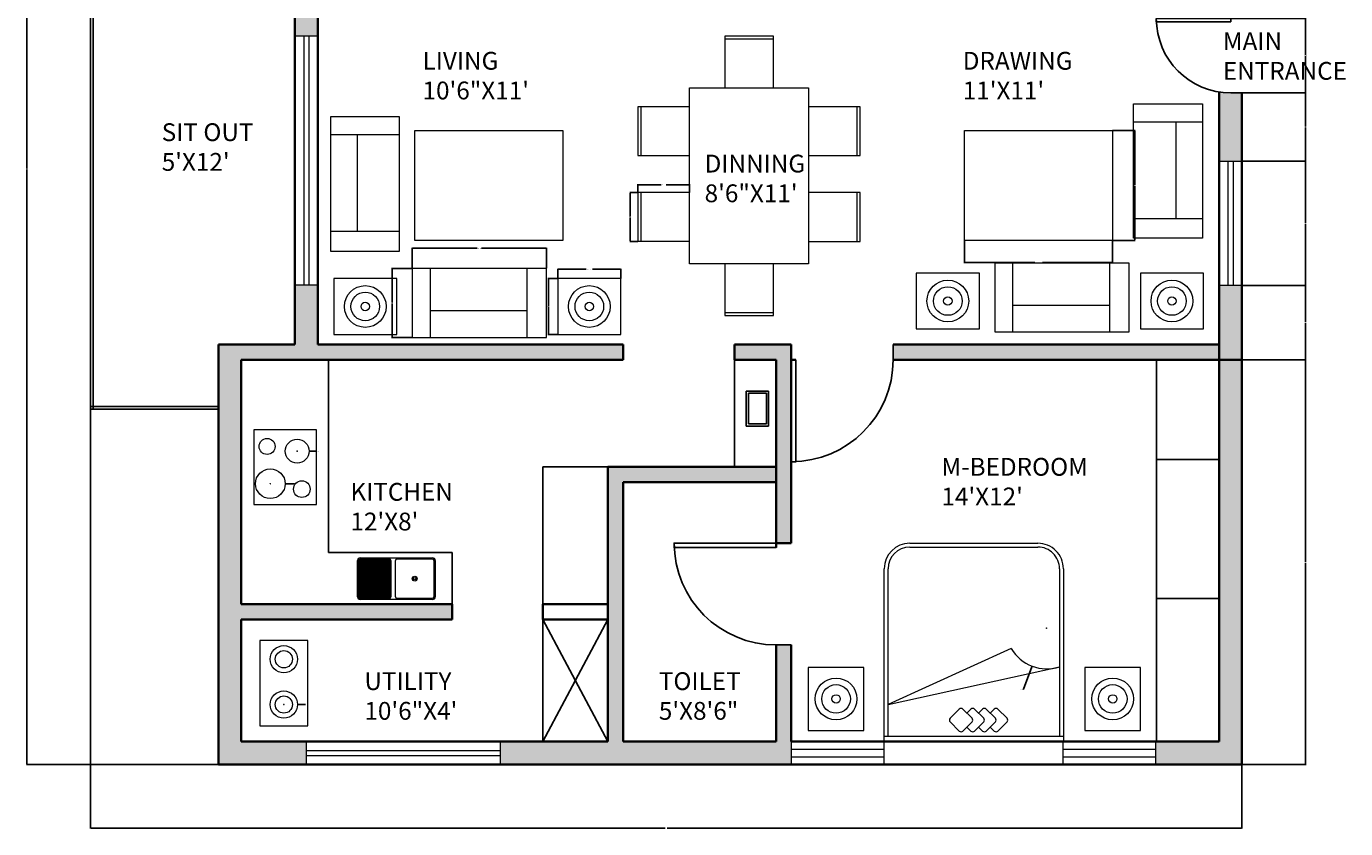
# Model space of a CAD drawing. Units: inches. Extents: x 2764 to 3282, y 1588 to 2106.
# Tile 1 of 2: x 2764 to 3282, y 1588 to 1903. Entities that reach past the tile are written whole.
import ezdxf

# ---------------------------------------------------------------- set-up
doc = ezdxf.new("R2010")
doc.units = ezdxf.units.IN
for name, color, linetype, lineweight in [('A-ANNO-DIMS', 2, 'Continuous', 18), ('A-ANNO-TEXT', 7, 'Continuous', 25), ('A-AREA-IDEN', 7, 'Continuous', 25), ('A-DOOR', 3, 'Continuous', 25), ('A-EQPM', 8, 'Continuous', 18), ('A-FIXT-PATT', 9, 'Continuous', 13), ('A-FLOR-CASE', 8, 'Continuous', 25), ('A-FLOR-FIXT', 9, 'Continuous', 18), ('A-FLOR-HRAL', 7, 'Continuous', 25), ('A-FURN', 8, 'Continuous', 18), ('A-GLAZ', 4, 'Continuous', 18), ('A-WALL', 7, 'Continuous', 35), ('A-WALL-PATT', 9, 'Continuous', 13)]:
    doc.layers.add(name, color=color, linetype=linetype, lineweight=lineweight)
doc.styles.get("Standard").update_dxf_attribs({"font": 'arial.ttf'})
doc.dimstyles.get("Standard").update_dxf_attribs({"dimtxt": 0.18, "dimasz": 0.18, "dimexe": 0.18, "dimexo": 0.0625, "dimgap": 0.09, "dimtad": 0, "dimtih": 1, "dimtoh": 1, "dimdec": 4, "dimzin": 0, "dimdsep": 46, "dimtxsty": 'Standard', "dimcen": 0.09, "dimadec": 0, "dimazin": 0, "dimtfac": 1, "dimtdec": 4, "dimtofl": 0, "dimtmove": 0, "dimatfit": 3, "dimfxl": 1, "dimtolj": 1, "dimtzin": 0, "dimarcsym": 0})

# ---------------------------------------------------------------- blocks, each defined once
blk = doc.blocks.new('*U2')
for p, q in [((0, 0), (0, -6)), ((40, 0), (40, -6))]:
    blk.add_line(p, q)
blk.add_lwpolyline([(0, 0), (0, 40), (1.75, 40), (1.75, 0)], close=True)
blk.add_arc((0, 0), 40, 0, 90)
blk = doc.blocks.new('SIDE-TABLE-WITH-LAMP')
for p, q in [((0, 21.93), (0, 0)), ((24.76, 21.93), (0, 21.93)), ((24.76, 0), (24.76, 21.93)), ((0, 0), (24.76, 0))]:
    blk.add_line(p, q)
for radius in [8.2, 5.62, 1.65]:
    blk.add_circle((12.38, 10.96), radius)
blk = doc.blocks.new('BED-DOUBLE')
for p, q in [((0, 70.34), (67.95, 70.34)), ((2.2, 70.34), (2.2, 0)), ((2.2, 68.84), (67.95, 68.84)), ((14.6, 68.84), (29.36, 1.5)), ((36.6, 20.47), (14.6, 68.84)), ((76.45, 60.34), (76.45, 10)), ((77.95, 60.34), (77.95, 10)), ((67.95, 0), (0, 0)), ((67.95, 1.5), (2.2, 1.5))]:
    blk.add_line(p, q)
blk.add_lwpolyline([(12.75, 40.88), (9.16, 44.46, 0.414214), (7.75, 44.46), (4.16, 40.88, 0.414214), (4.16, 39.46), (7.75, 35.88, 0.414214), (9.16, 35.88), (12.75, 39.46, 0.414214)], format="xyb", close=True)
for points in [[(5.75, 37.88), (4.16, 36.29, 0.414214), (4.16, 34.88), (7.75, 31.29, 0.414214), (9.16, 31.29), (12.75, 34.88, 0.414214), (12.75, 36.29), (11.16, 37.88)], [(5.75, 33.29), (4.16, 31.7, 0.414214), (4.16, 30.29), (7.75, 26.7, 0.414214), (9.16, 26.7), (12.75, 30.29, 0.414214), (12.75, 31.7), (11.16, 33.29)], [(5.75, 28.7), (4.16, 27.12, 0.414214), (4.16, 25.7), (7.75, 22.12, 0.414214), (9.16, 22.12), (12.75, 25.7, 0.414214), (12.75, 27.12), (11.16, 28.7)]]:
    blk.add_lwpolyline(points, format="xyb")
for centre, radius, start, end in [((67.95, 60.34), 10, 0, 90), ((67.95, 60.34), 8.5, 0, 90), ((44.61, 6.58), 16.03, 119.9541, 198.4829), ((67.95, 10), 10, 270, 0), ((67.95, 10), 8.5, 270, 0)]:
    blk.add_arc(centre, radius, start, end)
blk = doc.blocks.new('SOFA-TWO-SEAT')
for p, q in [((0, 27.06), (0, 0)), ((52.76, 27.06), (0, 27.06)), ((7, 27.06), (7, 0)), ((45.05, 27.06), (45.05, 0)), ((52.76, 0), (52.76, 27.06)), ((7, 10.5), (45.05, 10.5)), ((0, 0), (52.76, 0))]:
    blk.add_line(p, q)
blk = doc.blocks.new('CHAIR-DINING')
for p, q in [((20.31, 19.17), (0, 19.17)), ((0, 19.17), (0, 0)), ((1.17, 19.17), (1.17, 0)), ((0, 0), (20.31, 0))]:
    blk.add_line(p, q)
blk = doc.blocks.new('TABLE-COFFEE')
for p, q in [((0, 43.23), (58.08, 43.23)), ((0, 0), (0, 43.23)), ((58.08, 43.23), (58.08, 0)), ((58.08, 0), (0, 0))]:
    blk.add_line(p, q)
blk = doc.blocks.new('*D8')
at = {"layer": 'A-ANNO-DIMS', "color": 0, "lineweight": -2, "transparency": 16777216}
for p, q in [((2972.96, 1804.15), (2972.96, 1807.98)), ((2973.14, 1807.8), (2984.09, 1807.8)), ((2997.54, 1807.8), (2986.6, 1807.8)), ((2997.72, 1804.15), (2997.72, 1807.98))]:
    blk.add_line(p, q, dxfattribs=at)
at = {"layer": 'A-ANNO-DIMS', "color": 0, "transparency": 16777216}
for points in [[(2973.14, 1807.83), (2973.14, 1807.77), (2972.96, 1807.8)], [(2997.54, 1807.83), (2997.54, 1807.77), (2997.72, 1807.8)]]:
    blk.add_solid(points, dxfattribs=at)
at = {"layer": 'Defpoints', "color": 0, "transparency": 16777216}
for p in [(2972.96, 1804.09), (2997.72, 1807.8), (2997.72, 1804.09)]:
    blk.add_point(p, dxfattribs=at)
at = {"layer": 'A-ANNO-DIMS', "color": 0, "transparency": 16777216, "insert": (2985.34, 1807.8), "char_height": 0.18, "attachment_point": 5}
blk.add_mtext('\\A1;END TABLE 25 TYP.', dxfattribs=at)
blk = doc.blocks.new('*D9')
at = {"layer": 'A-ANNO-DIMS', "color": 0, "lineweight": -2, "transparency": 16777216}
for p, q in [((2972.9, 1804.09), (2969.07, 1804.09)), ((2969.25, 1803.91), (2969.25, 1793.31)), ((2969.25, 1782.34), (2969.25, 1792.95)), ((2972.9, 1782.16), (2969.07, 1782.16))]:
    blk.add_line(p, q, dxfattribs=at)
at = {"layer": 'A-ANNO-DIMS', "color": 0, "transparency": 16777216}
for points in [[(2969.22, 1803.91), (2969.28, 1803.91), (2969.25, 1804.09)], [(2969.22, 1782.34), (2969.28, 1782.34), (2969.25, 1782.16)]]:
    blk.add_solid(points, dxfattribs=at)
at = {"layer": 'Defpoints', "color": 0, "transparency": 16777216}
for p in [(2969.25, 1804.09), (2972.96, 1804.09), (2972.96, 1782.16)]:
    blk.add_point(p, dxfattribs=at)
at = {"layer": 'A-ANNO-DIMS', "color": 0, "transparency": 16777216, "insert": (2969.25, 1793.13), "char_height": 0.18, "attachment_point": 5}
blk.add_mtext('\\A1;22 TYP.', dxfattribs=at)
blk = doc.blocks.new('*D12')
at = {"layer": 'A-ANNO-DIMS', "color": 0, "lineweight": -2, "transparency": 16777216}
for p, q in [((3132.73, 1819.03), (3132.73, 1810.2)), ((3190.81, 1819.03), (3190.81, 1810.2)), ((3132.91, 1810.38), (3160.26, 1810.38)), ((3190.63, 1810.38), (3163.27, 1810.38))]:
    blk.add_line(p, q, dxfattribs=at)
at = {"layer": 'A-ANNO-DIMS', "color": 0, "transparency": 16777216}
for points in [[(3132.91, 1810.41), (3132.91, 1810.35), (3132.73, 1810.38)], [(3190.63, 1810.41), (3190.63, 1810.35), (3190.81, 1810.38)]]:
    blk.add_solid(points, dxfattribs=at)
at = {"layer": 'Defpoints', "color": 0, "transparency": 16777216}
for p in [(3132.73, 1819.09), (3190.81, 1819.09), (3190.81, 1810.38)]:
    blk.add_point(p, dxfattribs=at)
at = {"layer": 'A-ANNO-DIMS', "color": 0, "transparency": 16777216, "insert": (3161.77, 1810.38), "char_height": 0.18, "attachment_point": 5}
blk.add_mtext('\\A1;COFFEE TABLE 58 TYP.', dxfattribs=at)
blk = doc.blocks.new('*D13')
at = {"layer": 'A-ANNO-DIMS', "color": 0, "lineweight": -2, "transparency": 16777216}
for p, q in [((3190.87, 1862.32), (3199.7, 1862.32)), ((3199.52, 1862.14), (3199.52, 1840.89)), ((3199.52, 1819.27), (3199.52, 1840.52)), ((3190.87, 1819.09), (3199.7, 1819.09))]:
    blk.add_line(p, q, dxfattribs=at)
at = {"layer": 'A-ANNO-DIMS', "color": 0, "transparency": 16777216}
for points in [[(3199.49, 1862.14), (3199.55, 1862.14), (3199.52, 1862.32)], [(3199.49, 1819.27), (3199.55, 1819.27), (3199.52, 1819.09)]]:
    blk.add_solid(points, dxfattribs=at)
at = {"layer": 'Defpoints', "color": 0, "transparency": 16777216}
for p in [(3190.81, 1862.32), (3199.52, 1862.32), (3190.81, 1819.09)]:
    blk.add_point(p, dxfattribs=at)
at = {"layer": 'A-ANNO-DIMS', "color": 0, "transparency": 16777216, "insert": (3199.52, 1840.71), "char_height": 0.18, "attachment_point": 5}
blk.add_mtext('\\A1;43 TYP.', dxfattribs=at)
blk = doc.blocks.new('*D14')
at = {"layer": 'A-ANNO-DIMS', "color": 0, "lineweight": -2, "transparency": 16777216}
for p, q in [((2915.77, 1808.12), (2915.77, 1816.15)), ((2915.95, 1815.97), (2941.24, 1815.97)), ((2968.35, 1815.97), (2943.05, 1815.97)), ((2968.53, 1808.12), (2968.53, 1816.15))]:
    blk.add_line(p, q, dxfattribs=at)
at = {"layer": 'A-ANNO-DIMS', "color": 0, "transparency": 16777216}
for points in [[(2915.95, 1816), (2915.95, 1815.94), (2915.77, 1815.97)], [(2968.35, 1816), (2968.35, 1815.94), (2968.53, 1815.97)]]:
    blk.add_solid(points, dxfattribs=at)
at = {"layer": 'Defpoints', "color": 0, "transparency": 16777216}
for p in [(2968.53, 1815.97), (2915.77, 1808.06), (2968.53, 1808.06)]:
    blk.add_point(p, dxfattribs=at)
at = {"layer": 'A-ANNO-DIMS', "color": 0, "transparency": 16777216, "insert": (2942.15, 1815.97), "char_height": 0.18, "attachment_point": 5}
blk.add_mtext('\\A1;SOFA 53 TYP.', dxfattribs=at)
blk = doc.blocks.new('*D15')
at = {"layer": 'A-ANNO-DIMS', "color": 0, "lineweight": -2, "transparency": 16777216}
for p, q in [((2915.71, 1808.06), (2907.68, 1808.06)), ((2907.86, 1807.88), (2907.86, 1794.71)), ((2907.86, 1781.18), (2907.86, 1794.35)), ((2915.71, 1781), (2907.68, 1781))]:
    blk.add_line(p, q, dxfattribs=at)
at = {"layer": 'A-ANNO-DIMS', "color": 0, "transparency": 16777216}
for points in [[(2907.83, 1807.88), (2907.89, 1807.88), (2907.86, 1808.06)], [(2907.83, 1781.18), (2907.89, 1781.18), (2907.86, 1781)]]:
    blk.add_solid(points, dxfattribs=at)
at = {"layer": 'Defpoints', "color": 0, "transparency": 16777216}
for p in [(2907.86, 1808.06), (2915.77, 1808.06), (2915.77, 1781)]:
    blk.add_point(p, dxfattribs=at)
at = {"layer": 'A-ANNO-DIMS', "color": 0, "transparency": 16777216, "insert": (2907.86, 1794.53), "char_height": 0.18, "attachment_point": 5}
blk.add_mtext('\\A1;27 TYP.', dxfattribs=at)
blk = doc.blocks.new('*D16')
at = {"layer": 'A-ANNO-DIMS', "color": 0, "lineweight": -2, "transparency": 16777216}
for p, q in [((3004.42, 1837.95), (3004.42, 1841.12)), ((3004.6, 1840.94), (3013.62, 1840.94)), ((3024.55, 1840.94), (3015.52, 1840.94)), ((3024.73, 1837.95), (3024.73, 1841.12))]:
    blk.add_line(p, q, dxfattribs=at)
at = {"layer": 'A-ANNO-DIMS', "color": 0, "transparency": 16777216}
for points in [[(3004.6, 1840.97), (3004.6, 1840.91), (3004.42, 1840.94)], [(3024.55, 1840.97), (3024.55, 1840.91), (3024.73, 1840.94)]]:
    blk.add_solid(points, dxfattribs=at)
at = {"layer": 'Defpoints', "color": 0, "transparency": 16777216}
for p in [(3024.73, 1840.94), (3004.42, 1837.89), (3024.73, 1837.89)]:
    blk.add_point(p, dxfattribs=at)
at = {"layer": 'A-ANNO-DIMS', "color": 0, "transparency": 16777216, "insert": (3014.57, 1840.94), "char_height": 0.18, "attachment_point": 5}
blk.add_mtext('\\A1;CHAIR 20 TYP.', dxfattribs=at)
blk = doc.blocks.new('*D17')
at = {"layer": 'A-ANNO-DIMS', "color": 0, "lineweight": -2, "transparency": 16777216}
for p, q in [((3004.35, 1837.89), (3001.19, 1837.89)), ((3001.37, 1837.71), (3001.37, 1828.49)), ((3001.37, 1818.9), (3001.37, 1828.12)), ((3004.35, 1818.72), (3001.19, 1818.72))]:
    blk.add_line(p, q, dxfattribs=at)
at = {"layer": 'A-ANNO-DIMS', "color": 0, "transparency": 16777216}
for points in [[(3001.34, 1837.71), (3001.4, 1837.71), (3001.37, 1837.89)], [(3001.34, 1818.9), (3001.4, 1818.9), (3001.37, 1818.72)]]:
    blk.add_solid(points, dxfattribs=at)
at = {"layer": 'Defpoints', "color": 0, "transparency": 16777216}
for p in [(3001.37, 1837.89), (3004.42, 1837.89), (3004.42, 1818.72)]:
    blk.add_point(p, dxfattribs=at)
at = {"layer": 'A-ANNO-DIMS', "color": 0, "transparency": 16777216, "insert": (3001.37, 1828.31), "char_height": 0.18, "attachment_point": 5}
blk.add_mtext('\\A1;19 TYP.', dxfattribs=at)
blk = doc.blocks.new('*D18')
at = {"layer": 'A-ANNO-DIMS', "color": 0, "lineweight": -2, "transparency": 16777216}
for p, q in [((2789.46, 1752.72), (2789.46, 1587.96)), ((3241.66, 1613.08), (3241.66, 1587.96)), ((2789.64, 1588.14), (3015.16, 1588.14)), ((3241.48, 1588.14), (3015.96, 1588.14))]:
    blk.add_line(p, q, dxfattribs=at)
at = {"layer": 'A-ANNO-DIMS', "color": 0, "transparency": 16777216}
for points in [[(2789.64, 1588.17), (2789.64, 1588.11), (2789.46, 1588.14)], [(3241.48, 1588.17), (3241.48, 1588.11), (3241.66, 1588.14)]]:
    blk.add_solid(points, dxfattribs=at)
at = {"layer": 'Defpoints', "color": 0, "transparency": 16777216}
for p in [(2789.46, 1752.79), (3241.66, 1613.14), (3241.66, 1588.14)]:
    blk.add_point(p, dxfattribs=at)
at = {"layer": 'A-ANNO-DIMS', "color": 0, "transparency": 16777216, "insert": (3015.56, 1588.14), "char_height": 0.18, "attachment_point": 5}
blk.add_mtext('\\A1;452.2', dxfattribs=at)
blk = doc.blocks.new('*D19')
at = {"layer": 'A-ANNO-DIMS', "color": 0, "lineweight": -2, "transparency": 16777216}
for p, q in [((2839.6, 2081.14), (2764.28, 2081.14)), ((2764.46, 2080.96), (2764.46, 1847.33)), ((2764.46, 1613.32), (2764.46, 1846.96)), ((2839.6, 1613.14), (2764.28, 1613.14))]:
    blk.add_line(p, q, dxfattribs=at)
at = {"layer": 'A-ANNO-DIMS', "color": 0, "transparency": 16777216}
for points in [[(2764.43, 2080.96), (2764.49, 2080.96), (2764.46, 2081.14)], [(2764.43, 1613.32), (2764.49, 1613.32), (2764.46, 1613.14)]]:
    blk.add_solid(points, dxfattribs=at)
at = {"layer": 'Defpoints', "color": 0, "transparency": 16777216}
for p in [(2764.46, 2081.14), (2839.66, 2081.14), (2839.66, 1613.14)]:
    blk.add_point(p, dxfattribs=at)
at = {"layer": 'A-ANNO-DIMS', "color": 0, "transparency": 16777216, "insert": (2764.46, 1847.14), "char_height": 0.18, "attachment_point": 5}
blk.add_mtext('\\A1;468', dxfattribs=at)
blk = doc.blocks.new('*D30')
at = {"layer": 'A-ANNO-DIMS', "color": 0, "lineweight": -2, "transparency": 16777216}
for p, q in [((3241.72, 1772.14), (3266.84, 1772.14)), ((3266.66, 1771.96), (3266.66, 1692.83)), ((3266.66, 1613.32), (3266.66, 1692.46)), ((3241.72, 1613.14), (3266.84, 1613.14))]:
    blk.add_line(p, q, dxfattribs=at)
at = {"layer": 'A-ANNO-DIMS', "color": 0, "transparency": 16777216}
for points in [[(3266.63, 1771.96), (3266.69, 1771.96), (3266.66, 1772.14)], [(3266.63, 1613.32), (3266.69, 1613.32), (3266.66, 1613.14)]]:
    blk.add_solid(points, dxfattribs=at)
at = {"layer": 'Defpoints', "color": 0, "transparency": 16777216}
for p in [(3241.66, 1772.14), (3266.66, 1772.14), (3241.66, 1613.14)]:
    blk.add_point(p, dxfattribs=at)
at = {"layer": 'A-ANNO-DIMS', "color": 0, "transparency": 16777216, "insert": (3266.66, 1692.64), "char_height": 0.18, "attachment_point": 5}
blk.add_mtext('\\A1;159', dxfattribs=at)
blk = doc.blocks.new('*D31')
at = {"layer": 'A-ANNO-DIMS', "color": 0, "lineweight": -2, "transparency": 16777216}
for p, q in [((3241.72, 1801.31), (3266.84, 1801.31)), ((3266.66, 1801.13), (3266.66, 1786.91)), ((3266.66, 1772.32), (3266.66, 1786.55)), ((3241.72, 1772.14), (3266.84, 1772.14))]:
    blk.add_line(p, q, dxfattribs=at)
at = {"layer": 'A-ANNO-DIMS', "color": 0, "transparency": 16777216}
for points in [[(3266.63, 1801.13), (3266.69, 1801.13), (3266.66, 1801.31)], [(3266.63, 1772.32), (3266.69, 1772.32), (3266.66, 1772.14)]]:
    blk.add_solid(points, dxfattribs=at)
at = {"layer": 'Defpoints', "color": 0, "transparency": 16777216}
for p in [(3241.66, 1801.31), (3266.66, 1801.31), (3241.66, 1772.14)]:
    blk.add_point(p, dxfattribs=at)
at = {"layer": 'A-ANNO-DIMS', "color": 0, "transparency": 16777216, "insert": (3266.66, 1786.73), "char_height": 0.18, "attachment_point": 5}
blk.add_mtext('\\A1;29.17', dxfattribs=at)
blk = doc.blocks.new('*D32')
at = {"layer": 'A-ANNO-DIMS', "color": 0, "lineweight": -2, "transparency": 16777216}
for p, q in [((3241.72, 1850.23), (3266.84, 1850.23)), ((3266.66, 1850.05), (3266.66, 1825.95)), ((3266.66, 1801.49), (3266.66, 1825.59)), ((3241.72, 1801.31), (3266.84, 1801.31))]:
    blk.add_line(p, q, dxfattribs=at)
at = {"layer": 'A-ANNO-DIMS', "color": 0, "transparency": 16777216}
for points in [[(3266.63, 1850.05), (3266.69, 1850.05), (3266.66, 1850.23)], [(3266.63, 1801.49), (3266.69, 1801.49), (3266.66, 1801.31)]]:
    blk.add_solid(points, dxfattribs=at)
at = {"layer": 'Defpoints', "color": 0, "transparency": 16777216}
for p in [(3241.66, 1850.23), (3266.66, 1850.23), (3241.66, 1801.31)]:
    blk.add_point(p, dxfattribs=at)
at = {"layer": 'A-ANNO-DIMS', "color": 0, "transparency": 16777216, "insert": (3266.66, 1825.77), "char_height": 0.18, "attachment_point": 5}
blk.add_mtext('\\A1;48.91', dxfattribs=at)
blk = doc.blocks.new('*D33')
at = {"layer": 'A-ANNO-DIMS', "color": 0, "lineweight": -2, "transparency": 16777216}
for p, q in [((3241.72, 1877.01), (3266.84, 1877.01)), ((3266.66, 1876.83), (3266.66, 1863.8)), ((3266.66, 1850.41), (3266.66, 1863.44)), ((3241.72, 1850.23), (3266.84, 1850.23))]:
    blk.add_line(p, q, dxfattribs=at)
at = {"layer": 'A-ANNO-DIMS', "color": 0, "transparency": 16777216}
for points in [[(3266.63, 1876.83), (3266.69, 1876.83), (3266.66, 1877.01)], [(3266.63, 1850.41), (3266.69, 1850.41), (3266.66, 1850.23)]]:
    blk.add_solid(points, dxfattribs=at)
at = {"layer": 'Defpoints', "color": 0, "transparency": 16777216}
for p in [(3241.66, 1877.01), (3266.66, 1877.01), (3241.66, 1850.23)]:
    blk.add_point(p, dxfattribs=at)
at = {"layer": 'A-ANNO-DIMS', "color": 0, "transparency": 16777216, "insert": (3266.66, 1863.62), "char_height": 0.18, "attachment_point": 5}
blk.add_mtext('\\A1;26.78', dxfattribs=at)
blk = doc.blocks.new('*D34')
at = {"layer": 'A-ANNO-DIMS', "color": 0, "lineweight": -2, "transparency": 16777216}
for p, q in [((3241.72, 1906.27), (3266.84, 1906.27)), ((3266.66, 1906.09), (3266.66, 1891.82)), ((3266.66, 1877.19), (3266.66, 1891.46)), ((3241.72, 1877.01), (3266.84, 1877.01))]:
    blk.add_line(p, q, dxfattribs=at)
at = {"layer": 'A-ANNO-DIMS', "color": 0, "transparency": 16777216}
for points in [[(3266.63, 1906.09), (3266.69, 1906.09), (3266.66, 1906.27)], [(3266.63, 1877.19), (3266.69, 1877.19), (3266.66, 1877.01)]]:
    blk.add_solid(points, dxfattribs=at)
at = {"layer": 'Defpoints', "color": 0, "transparency": 16777216}
for p in [(3241.66, 1906.27), (3266.66, 1906.27), (3241.66, 1877.01)]:
    blk.add_point(p, dxfattribs=at)
at = {"layer": 'A-ANNO-DIMS', "color": 0, "transparency": 16777216, "insert": (3266.66, 1891.64), "char_height": 0.18, "attachment_point": 5}
blk.add_mtext('\\A1;29.253', dxfattribs=at)
blk = doc.blocks.new('*D38')
at = {"layer": 'A-ANNO-DIMS', "color": 0, "lineweight": -2, "transparency": 16777216}
for p, q in [((3164.84, 1666.75), (3165.02, 1666.75)), ((3164.93, 1666.66), (3164.93, 1666.84)), ((3155.83, 1642.77), (3159.18, 1651.6)), ((3155.65, 1642.77), (3155.83, 1642.77))]:
    blk.add_line(p, q, dxfattribs=at)
at = {"layer": 'A-ANNO-DIMS', "color": 0, "transparency": 16777216}
blk.add_solid([(3159.15, 1651.61), (3159.21, 1651.59), (3159.24, 1651.77)], dxfattribs=at)
at = {"layer": 'Defpoints', "color": 0, "transparency": 16777216}
for p in [(3164.93, 1666.75), (3159.24, 1651.77)]:
    blk.add_point(p, dxfattribs=at)
at = {"layer": 'A-ANNO-DIMS', "color": 0, "transparency": 16777216, "insert": (3154.91, 1642.77), "char_height": 0.18, "attachment_point": 5}
blk.add_mtext('\\A1;3X R16.028', dxfattribs=at)
blk = doc.blocks.new('*D43')
at = {"layer": 'A-ANNO-DIMS', "color": 0, "lineweight": -2, "transparency": 16777216}
for p, q in [((2859.97, 1723.49), (2860.15, 1723.49)), ((2860.06, 1723.4), (2860.06, 1723.58)), ((2869.39, 1723.49), (2866.07, 1723.49))]:
    blk.add_line(p, q, dxfattribs=at)
at = {"layer": 'A-ANNO-DIMS', "color": 0, "transparency": 16777216}
blk.add_solid([(2866.07, 1723.52), (2866.07, 1723.46), (2865.89, 1723.49)], dxfattribs=at)
at = {"layer": 'Defpoints', "color": 0, "transparency": 16777216}
for p in [(2854.23, 1723.49), (2865.89, 1723.49)]:
    blk.add_point(p, dxfattribs=at)
at = {"layer": 'A-ANNO-DIMS', "color": 0, "transparency": 16777216, "insert": (2869.95, 1723.49), "char_height": 0.18, "attachment_point": 5}
blk.add_mtext('\\A1;∅11.663', dxfattribs=at)
blk = doc.blocks.new('*D44')
at = {"layer": 'A-ANNO-DIMS', "color": 0, "lineweight": -2, "transparency": 16777216}
for p, q in [((2865.28, 1636.71), (2865.46, 1636.71)), ((2865.37, 1636.62), (2865.37, 1636.8)), ((2873.91, 1636.71), (2870.89, 1636.71))]:
    blk.add_line(p, q, dxfattribs=at)
at = {"layer": 'A-ANNO-DIMS', "color": 0, "transparency": 16777216}
blk.add_solid([(2870.89, 1636.74), (2870.89, 1636.68), (2870.71, 1636.71)], dxfattribs=at)
at = {"layer": 'Defpoints', "color": 0, "transparency": 16777216}
for p in [(2860.03, 1636.71), (2870.71, 1636.71)]:
    blk.add_point(p, dxfattribs=at)
at = {"layer": 'A-ANNO-DIMS', "color": 0, "transparency": 16777216, "insert": (2874.66, 1636.71), "char_height": 0.18, "attachment_point": 5}
blk.add_mtext('\\A1;2X ∅10.675', dxfattribs=at)
blk = doc.blocks.new('*D45')
at = {"layer": 'A-ANNO-DIMS', "color": 0, "lineweight": -2, "transparency": 16777216}
for p, q in [((2870.5, 1736.28), (2870.68, 1736.28)), ((2870.59, 1736.19), (2870.59, 1736.37)), ((2878.1, 1736.28), (2875.46, 1736.28))]:
    blk.add_line(p, q, dxfattribs=at)
at = {"layer": 'A-ANNO-DIMS', "color": 0, "transparency": 16777216}
blk.add_solid([(2875.46, 1736.31), (2875.46, 1736.25), (2875.28, 1736.28)], dxfattribs=at)
at = {"layer": 'Defpoints', "color": 0, "transparency": 16777216}
for p in [(2865.89, 1736.28), (2875.28, 1736.28)]:
    blk.add_point(p, dxfattribs=at)
at = {"layer": 'A-ANNO-DIMS', "color": 0, "transparency": 16777216, "insert": (2878.59, 1736.28), "char_height": 0.18, "attachment_point": 5}
blk.add_mtext('\\A1;∅9.388', dxfattribs=at)

msp = doc.modelspace()

# ---------------------------------------------------------------- hatches: boundary and pattern name
at = {"layer": 'A-FIXT-PATT'}
h = msp.add_hatch(dxfattribs=at)
h.set_pattern_fill('ANSI31', color=256, scale=0.1574803, angle=-45, style=0)
h.paths.add_polyline_path([(2907.3596, 1693.3563), (2907.3499, 1693.4539), (2907.3215, 1693.5477), (2907.2753, 1693.6341), (2907.2131, 1693.7099), (2907.1373, 1693.7721), (2907.0509, 1693.8183), (2906.9571, 1693.8467), (2906.8596, 1693.8563), (2895.2983, 1693.8563), (2895.2007, 1693.8467), (2895.1069, 1693.8183), (2895.0205, 1693.7721), (2894.9447, 1693.7099), (2894.8825, 1693.6341), (2894.8363, 1693.5477), (2894.8079, 1693.4539), (2894.7983, 1693.3563), (2894.7983, 1678.9912), (2894.8079, 1678.8936), (2894.8363, 1678.7998), (2894.8825, 1678.7134), (2894.9447, 1678.6376), (2895.0205, 1678.5755), (2895.1069, 1678.5292), (2895.2007, 1678.5008), (2895.2983, 1678.4912), (2906.8596, 1678.4912), (2906.9571, 1678.5008), (2907.0509, 1678.5292), (2907.1373, 1678.5755), (2907.2131, 1678.6376), (2907.2753, 1678.7134), (2907.3215, 1678.7998), (2907.3499, 1678.8936), (2907.3596, 1678.9912)])
at = {"layer": 'A-WALL-PATT'}
h = msp.add_hatch(color=256, dxfattribs=at)
h.dxf.hatch_style = 1
h.paths.add_polyline_path([(2848.6606, 1954.2983), (2839.6606, 1954.2983), (2839.6606, 1922.1439), (2848.6606, 1922.1439)])
h.paths.add_polyline_path([(3004.6606, 1928.1439), (2999.2578, 1928.1439), (2963.2391, 1928.1439), (2848.6606, 1928.1439), (2848.6606, 1922.1439), (3004.6606, 1922.1439)])
h.paths.add_polyline_path([(3241.6606, 1954.2983), (3232.6606, 1954.2983), (3232.6606, 1928.1439), (3070.6606, 1928.1439), (3070.6606, 1922.1439), (3232.6606, 1922.1439), (3232.6606, 1906.2651), (3237.2727, 1906.2651), (3241.6606, 1906.2651)])
h.paths.add_polyline_path([(2878.6606, 1922.1439), (2869.6606, 1922.1439), (2869.6606, 1899.4014), (2878.6606, 1899.4014)])
h = msp.add_hatch(color=256, dxfattribs=at)
h.dxf.hatch_style = 1
h.paths.add_polyline_path([(3064.6606, 1778.1439), (3042.3076, 1778.1439), (3042.3076, 1772.1439), (3058.6606, 1772.1439), (3058.6606, 1700.1439), (3064.6606, 1700.1439)])
h.paths.add_polyline_path([(3232.6606, 1778.1439), (3104.6606, 1778.1439), (3104.6606, 1772.1439), (3232.6606, 1772.1439)])
h.paths.add_polyline_path([(3241.6606, 1801.315), (3232.6606, 1801.315), (3232.6606, 1778.1439), (3232.6606, 1772.1439), (3241.6606, 1772.1439), (3241.6606, 1778.1439)])
h.paths.add_polyline_path([(3241.6606, 1877.0118), (3237.2727, 1877.0118, -0.03960023), (3232.6606, 1877.3777), (3232.6606, 1850.2298), (3241.6606, 1850.2298)])
h = msp.add_hatch(color=256, dxfattribs=at)
h.dxf.hatch_style = 1
h.paths.add_polyline_path([(3064.6606, 1622.1439), (3064.6606, 1660.1439), (3058.6606, 1660.1439), (3058.6606, 1622.1439), (2998.6606, 1622.1439), (2998.6606, 1724.1439), (3058.6606, 1724.1439), (3058.6606, 1730.1439), (2992.6606, 1730.1439), (2992.6606, 1670.1439), (2992.6606, 1622.1439), (2950.4987, 1622.1439), (2950.4987, 1613.1439), (3064.6606, 1613.1439)])
h.paths.add_polyline_path([(2848.6606, 1772.1439), (2992.6606, 1772.1439), (2998.6606, 1772.1439), (2998.6606, 1778.1439), (2878.6606, 1778.1439), (2878.6606, 1801.4507), (2869.6606, 1801.4507), (2869.6606, 1778.1439), (2839.6606, 1778.1439), (2839.6606, 1613.1439), (2874.134, 1613.1439), (2874.134, 1622.1439), (2848.6606, 1622.1439), (2848.6606, 1670.1439), (2931.4932, 1670.1439), (2931.4932, 1676.1439), (2848.6606, 1676.1439)])
h = msp.add_hatch(color=256, dxfattribs=at)
h.dxf.hatch_style = 1
h.paths.add_polyline_path([(3241.6606, 1772.1439), (3232.6606, 1772.1439), (3232.6606, 1622.1439), (3207.8789, 1622.1439), (3207.8789, 1613.1439), (3241.6606, 1613.1439)])

# ---------------------------------------------------------------- linework, layer by layer
at = {"layer": 'A-EQPM'}
for p, q in [((2853.554, 1744.6743), (2853.554, 1715.2995)), ((2878.2313, 1744.6743), (2853.554, 1744.6743)), ((2878.2313, 1715.2995), (2878.2313, 1744.6743)), ((2853.554, 1715.2995), (2878.2313, 1715.2995)), ((2855.9931, 1661.9011), (2855.9931, 1628.3814)), ((2874.7482, 1661.9011), (2855.9931, 1661.9011)), ((2874.7482, 1628.3814), (2874.7482, 1661.9011)), ((2855.9931, 1628.3814), (2874.7482, 1628.3814))]:
    msp.add_line(p, q, dxfattribs=at)
for centre, radius in [((2858.7793, 1738.132), 3.1292), ((2870.585, 1736.2842), 4.6938), ((2860.0594, 1723.4916), 5.8317), ((2872.4341, 1721.3595), 3.2715), ((2865.3707, 1654.5208), 5.3375), ((2865.3707, 1654.5208), 3.3847), ((2865.3707, 1636.7133), 5.3375), ((2865.3707, 1636.7133), 3.3847)]:
    msp.add_circle(centre, radius, dxfattribs=at)
at = {"layer": 'A-FLOR-CASE'}
for p, q in [((2882.949, 1772.1439), (2882.949, 1696.4415)), ((3042.3076, 1772.1439), (3042.3076, 1730.1439)), ((3208.0335, 1772.1439), (3208.0335, 1622.1439)), ((3046.9623, 1759.8644), (3055.7662, 1759.8644)), ((3046.9623, 1746.1059), (3046.9623, 1759.8644)), ((3047.8685, 1759.0158), (3047.8685, 1747.0623)), ((3054.9635, 1759.0158), (3047.8685, 1759.0158)), ((3054.9635, 1747.0623), (3054.9635, 1759.0158)), ((3055.7662, 1759.8644), (3055.7662, 1746.1059)), ((3055.7662, 1746.1059), (3046.9623, 1746.1059)), ((3047.8685, 1747.0623), (3054.9635, 1747.0623)), ((3208.0335, 1733.064), (3232.6606, 1733.064)), ((2992.6606, 1730.1439), (2967.1121, 1730.1439)), ((2967.1121, 1730.1439), (2967.1121, 1622.1439)), ((2882.949, 1696.4415), (2931.4932, 1696.4415)), ((2931.4932, 1696.4415), (2931.4932, 1676.1439)), ((3208.0335, 1678.3245), (3232.6606, 1678.3245)), ((2967.1121, 1670.1439), (2992.6606, 1622.1439)), ((2992.6606, 1670.1439), (2967.1121, 1622.1439))]:
    msp.add_line(p, q, dxfattribs=at)
at = {"layer": 'A-FLOR-FIXT'}
for p, q in [((2895.2983, 1694.3563), (2923.8137, 1694.3563)), ((2894.2983, 1678.9912), (2894.2983, 1693.3563)), ((2894.7983, 1678.9912), (2894.7983, 1693.3563)), ((2895.2983, 1693.8563), (2906.8596, 1693.8563)), ((2907.3596, 1693.3563), (2907.3596, 1678.9912)), ((2909.2051, 1678.9912), (2909.2051, 1693.3563)), ((2923.8137, 1693.8563), (2909.7051, 1693.8563)), ((2924.3137, 1693.3563), (2924.3137, 1678.9912)), ((2924.8137, 1693.3563), (2924.8137, 1678.9912)), ((2906.8596, 1678.4912), (2895.2983, 1678.4912)), ((2923.8137, 1677.9912), (2895.2983, 1677.9912)), ((2909.7051, 1678.4912), (2923.8137, 1678.4912))]:
    msp.add_line(p, q, dxfattribs=at)
for radius in [0.9807, 0.4807]:
    msp.add_circle((2916.7594, 1686.1738), radius, dxfattribs=at)
for centre, radius, start, end in [((2895.2983, 1693.3563), 1, 90, 180), ((2923.8137, 1693.3563), 1, 0, 90), ((2895.2983, 1693.3563), 0.5, 90, 180), ((2906.8596, 1693.3563), 0.5, 0, 90), ((2909.7051, 1693.3563), 0.5, 90, 180), ((2923.8137, 1693.3563), 0.5, 0, 90), ((2895.2983, 1678.9912), 1, 180, 270), ((2895.2983, 1678.9912), 0.5, 180, 270), ((2906.8596, 1678.9912), 0.5, 270, 0), ((2909.7051, 1678.9912), 0.5, 180, 270), ((2923.8137, 1678.9912), 1, 270, 0), ((2923.8137, 1678.9912), 0.5, 270, 0)]:
    msp.add_arc(centre, radius, start, end, dxfattribs=at)
at = {"layer": 'A-FLOR-HRAL'}
for p, q in [((2789.4608, 1941.8045), (2789.4608, 1752.7872)), ((2790.4608, 1941.8045), (2790.4608, 1752.7872)), ((2789.4608, 1753.7872), (2839.6606, 1753.7872)), ((2789.4608, 1752.7872), (2839.6606, 1752.7872))]:
    msp.add_line(p, q, dxfattribs=at)
at = {"layer": 'A-FURN'}
for p, q in [((3024.7252, 1879.0759), (3071.3608, 1879.0759)), ((3024.7252, 1809.9221), (3024.7252, 1879.0759)), ((3071.3608, 1879.0759), (3071.3608, 1809.9221)), ((3071.3608, 1809.9221), (3024.7252, 1809.9221))]:
    msp.add_line(p, q, dxfattribs=at)
at = {"layer": 'A-GLAZ'}
for p, q in [((2869.6606, 1899.4014), (2878.6606, 1899.4014)), ((2873.1606, 1899.4014), (2873.1606, 1801.4507)), ((2875.1606, 1899.4014), (2875.1606, 1801.4507)), ((2878.6606, 1899.4014), (2878.6606, 1801.4507)), ((3232.6606, 1850.2298), (3241.6606, 1850.2298)), ((3236.1606, 1850.2298), (3236.1606, 1801.315)), ((3238.1606, 1850.2298), (3238.1606, 1801.315)), ((3241.6606, 1850.2298), (3241.6606, 1801.315)), ((2878.6606, 1801.4507), (2869.6606, 1801.4507)), ((3241.6606, 1801.315), (3232.6606, 1801.315)), ((2874.134, 1622.1439), (2874.134, 1613.1439)), ((2950.4987, 1613.1439), (2950.4987, 1622.1439)), ((3064.6606, 1622.1439), (3064.6606, 1613.1439)), ((3101.1753, 1613.1439), (3101.1753, 1622.1439)), ((3171.3642, 1622.1439), (3171.3642, 1613.1439)), ((3207.8789, 1613.1439), (3207.8789, 1622.1439)), ((2874.134, 1618.6439), (2950.4987, 1618.6439)), ((2874.134, 1616.6439), (2950.4987, 1616.6439)), ((3064.6606, 1619.1439), (3101.1753, 1619.1439)), ((3171.3642, 1619.1439), (3207.8789, 1619.1439)), ((2874.134, 1613.1439), (2950.4987, 1613.1439)), ((3064.6606, 1616.1439), (3101.1753, 1616.1439)), ((3064.6606, 1613.1439), (3101.1753, 1613.1439)), ((3171.3642, 1616.1439), (3207.8789, 1616.1439))]:
    msp.add_line(p, q, dxfattribs=at)
at = {"layer": 'A-WALL'}
for p, q in [((2869.6606, 1922.1439), (2869.6606, 1778.1439)), ((2878.6606, 1922.1439), (2878.6606, 1778.1439)), ((3232.6606, 1877.3777), (3232.6606, 1778.1439)), ((3241.6606, 1877.0118), (3241.6606, 1773.1439)), ((2869.6606, 1778.1439), (2839.6606, 1778.1439)), ((2839.6606, 1778.1439), (2839.6606, 1613.1439)), ((2998.6606, 1778.1439), (2878.6606, 1778.1439)), ((2998.6606, 1778.1439), (2998.6606, 1772.1439)), ((3042.3076, 1778.1439), (3042.3076, 1772.1439)), ((3064.6606, 1778.1439), (3042.3076, 1778.1439)), ((3064.6606, 1778.1439), (3064.6606, 1700.1439)), ((3232.6606, 1778.1439), (3104.6606, 1778.1439)), ((3232.6606, 1778.1439), (3232.6606, 1622.1439)), ((3241.6606, 1778.1439), (3241.6606, 1613.1439)), ((2848.6606, 1772.1439), (2848.6606, 1676.1439)), ((2992.6606, 1772.1439), (2848.6606, 1772.1439)), ((2998.6606, 1772.1439), (2992.6606, 1772.1439)), ((3058.6606, 1772.1439), (3042.3076, 1772.1439)), ((3058.6606, 1772.1439), (3058.6606, 1698.3939)), ((3066.4106, 1772.1439), (3064.6606, 1772.1439)), ((3241.6606, 1772.1439), (3104.6606, 1772.1439)), ((3058.6606, 1730.1439), (2992.6606, 1730.1439)), ((2992.6606, 1730.1439), (2992.6606, 1670.1439)), ((3058.6606, 1724.1439), (2998.6606, 1724.1439)), ((2998.6606, 1724.1439), (2998.6606, 1622.1439)), ((3064.6606, 1700.1439), (3058.6606, 1700.1439)), ((2931.4932, 1676.1439), (2848.6606, 1676.1439)), ((2931.4932, 1670.1439), (2931.4932, 1676.1439)), ((2992.6606, 1676.1439), (2967.1121, 1676.1439)), ((2967.1121, 1676.1439), (2967.1121, 1670.1439)), ((2848.6606, 1670.1439), (2848.6606, 1622.1439)), ((2931.4932, 1670.1439), (2848.6606, 1670.1439)), ((2992.6606, 1670.1439), (2967.1121, 1670.1439)), ((2992.6606, 1670.1439), (2992.6606, 1622.1439)), ((3058.6606, 1660.1439), (3058.6606, 1622.1439)), ((3064.6606, 1660.1439), (3064.6606, 1622.1439)), ((2992.6606, 1622.1439), (2848.6606, 1622.1439)), ((3058.6606, 1622.1439), (2998.6606, 1622.1439)), ((3232.6606, 1622.1439), (3064.6606, 1622.1439)), ((3241.6606, 1613.1439), (2839.6606, 1613.1439))]:
    msp.add_line(p, q, dxfattribs=at)

# ---------------------------------------------------------------- block references
at = {"layer": 'A-DOOR', "xscale": -0.731332392084942, "yscale": 0.731332392084942, "zscale": 0.731332392084942, "rotation": 90}
msp.add_blockref('*U2', (3237.2727, 1906.2651), dxfattribs=at)
at = {"layer": 'A-DOOR', "xscale": -1}
for p, rotation in [((3064.6606, 1772.1439), 180), ((3058.6606, 1700.1439), 90)]:
    msp.add_blockref('*U2', p, dxfattribs=dict(at, rotation=rotation))
at = {"layer": 'A-FURN'}
for name, p, rotation in [('CHAIR-DINING', (3038.552, 1899.3851), 270.0000000000017), ('CHAIR-DINING', (3091.6699, 1871.5587), 180), ('SOFA-TWO-SEAT', (2883.6809, 1867.577), 270.0000000000006), ('CHAIR-DINING', (3091.6699, 1837.8888), 180), ('CHAIR-DINING', (3057.7188, 1789.6129), 90.00000000000325), ('BED-DOUBLE', (3171.5122, 1622.1443), 90.00000000000136), ('SIDE-TABLE-WITH-LAMP', (3093.2052, 1626.5333), 90.00000000000561), ('SIDE-TABLE-WITH-LAMP', (3201.8591, 1626.5333), 90.00000000000328)]:
    msp.add_blockref(name, p, dxfattribs=dict(at, rotation=rotation))
for name, p in [('CHAIR-DINING', (3004.416, 1852.392)), ('TABLE-COFFEE', (2916.867, 1819.088)), ('TABLE-COFFEE', (3132.7272, 1819.088)), ('CHAIR-DINING', (3004.416, 1818.7221)), ('SOFA-TWO-SEAT', (3144.5657, 1783.1431)), ('SIDE-TABLE-WITH-LAMP', (2884.9565, 1782.1636)), ('SOFA-TWO-SEAT', (2915.77, 1780.998)), ('SIDE-TABLE-WITH-LAMP', (2972.9614, 1782.1636)), ('SIDE-TABLE-WITH-LAMP', (3113.7522, 1784.3087)), ('SIDE-TABLE-WITH-LAMP', (3201.7571, 1784.3087))]:
    msp.add_blockref(name, p, dxfattribs=at)
at = {"layer": 'A-FURN', "extrusion": (0, 0, -1), "zscale": -1, "rotation": 269.9999999999991}
msp.add_blockref('SOFA-TWO-SEAT', (-3226.1435, 1872.6817), dxfattribs=at)

# ---------------------------------------------------------------- texts
at = {"layer": 'A-ANNO-TEXT', "insert": (3234.1439, 1900.8724), "char_height": 7, "attachment_point": 1}
msp.add_mtext_dynamic_manual_height_columns('MAIN\\PENTRANCE', width=45.041222, gutter_width=12.5, heights=[0], dxfattribs=at)
at = {"layer": 'A-AREA-IDEN', "char_height": 7, "attachment_point": 1}
for s, insert in [('LIVING\\P10\'6"X11\'', (2919.8405, 1893.1656)), ("DRAWING\\P11'X11'", (3131.9906, 1893.1656)), ("SIT OUT\\P5'X12'", (2817.4103, 1865.1052)), ('DINNING\\P8\'6"X11\'', (3030.6201, 1852.7639)), ("M-BEDROOM\\P14'X12'", (3123.6185, 1733.6291)), ("KITCHEN\\P12'X8'", (2891.5208, 1723.7907)), ('UTILITY\\P10\'6"X4\'', (2897.0053, 1649.4058)), ('TOILET\\P5\'X8\'6"', (3012.6427, 1649.4058))]:
    msp.add_mtext_dynamic_manual_height_columns(s, width=45.041222, gutter_width=12.5, heights=[0], dxfattribs=dict(at, insert=insert))

# ---------------------------------------------------------------- dimensions: what is measured, and where the dimension line sits
at = {"layer": 'A-ANNO-DIMS'}
for base, p1, p2, override, picture, middle in [((2764.4608, 2081.1439), (2839.6606, 1613.1439), (2839.6606, 2081.1439), {"dimdec": 0, "dimlfac": 1, "dimrnd": 0, "dimzin": 0, "dimdsep": 46, "dimlunit": 2}, '*D19', (2764.4608, 1847.1439)), ((3266.6606, 1906.2651), (3241.6606, 1877.0118), (3241.6606, 1906.2651), {"dimdec": 3, "dimlfac": 1, "dimrnd": 0, "dimzin": 0, "dimdsep": 46, "dimlunit": 2}, '*D34', (3266.6606, 1891.6385)), ((3266.6606, 1877.0118), (3241.6606, 1850.2298), (3241.6606, 1877.0118), {"dimdec": 2, "dimlfac": 1, "dimrnd": 0, "dimzin": 0, "dimdsep": 46, "dimlunit": 2}, '*D33', (3266.6606, 1863.6208)), ((3266.6606, 1850.2298), (3241.6606, 1801.315), (3241.6606, 1850.2298), {"dimdec": 2, "dimlfac": 1, "dimrnd": 0, "dimzin": 0, "dimdsep": 46, "dimlunit": 2}, '*D32', (3266.6606, 1825.7724)), ((3266.6606, 1801.315), (3241.6606, 1772.1439), (3241.6606, 1801.315), {"dimdec": 2, "dimlfac": 1, "dimrnd": 0, "dimzin": 0, "dimdsep": 46, "dimlunit": 2}, '*D31', (3266.6606, 1786.7295)), ((3266.6606, 1772.1439), (3241.6606, 1613.1439), (3241.6606, 1772.1439), {"dimdec": 0, "dimlfac": 1, "dimrnd": 0, "dimzin": 0, "dimdsep": 46, "dimlunit": 2}, '*D30', (3266.6606, 1692.6439))]:
    dim = msp.add_linear_dim(base=base, p1=p1, p2=p2, angle=90, dimstyle='Standard', override=override, dxfattribs=at)
    dim.commit()
    dim.dimension.update_dxf_attribs({"geometry": picture, "text_midpoint": middle})
for base, p1, p2, picture, middle in [((3199.519, 1862.3222), (3190.807, 1819.0881), (3190.807, 1862.3222), '*D13', (3199.519, 1840.7052)), ((3001.3698, 1837.8893), (3004.4161, 1818.7217), (3004.4161, 1837.8893), '*D17', (3001.3698, 1828.3055)), ((2907.8563, 1808.0575), (2915.7697, 1780.9976), (2915.7697, 1808.0575), '*D15', (2907.8563, 1794.5276)), ((2969.2469, 1804.0901), (2972.9612, 1782.164), (2972.9612, 1804.0901), '*D9', (2969.2469, 1793.1271))]:
    dim = msp.add_linear_dim(base=base, p1=p1, p2=p2, angle=90, text='<> TYP.', dimstyle='Standard', override={"dimdec": 0, "dimlfac": 1, "dimrnd": 0, "dimzin": 0, "dimdsep": 46, "dimlunit": 2}, dxfattribs=at)
    dim.commit()
    dim.dimension.update_dxf_attribs({"geometry": picture, "text_midpoint": middle})
for base, p1, p2, text, picture, middle in [((3024.7252, 1840.9357), (3004.4161, 1837.8893), (3024.7252, 1837.8893), 'CHAIR <> TYP.', '*D16', (3014.5707, 1840.9357)), ((3190.807, 1810.3761), (3132.7269, 1819.0881), (3190.807, 1819.0881), 'COFFEE TABLE <> TYP.', '*D12', (3161.767, 1810.3761)), ((2968.526, 1815.971), (2915.7697, 1808.0575), (2968.526, 1808.0575), 'SOFA <> TYP.', '*D14', (2942.1479, 1815.971)), ((2997.7234, 1807.8045), (2972.9612, 1804.0901), (2997.7234, 1804.0901), 'END TABLE <> TYP.', '*D8', (2985.3423, 1807.8045))]:
    dim = msp.add_linear_dim(base=base, p1=p1, p2=p2, text=text, dimstyle='Standard', override={"dimdec": 0, "dimlfac": 1, "dimrnd": 0, "dimzin": 0, "dimdsep": 46, "dimlunit": 2}, dxfattribs=at)
    dim.commit()
    dim.dimension.update_dxf_attribs({"geometry": picture, "text_midpoint": middle})
dim = msp.add_linear_dim(base=(3241.6606, 1588.1439), p1=(2789.4608, 1752.7872), p2=(3241.6606, 1613.1439), dimstyle='Standard', override={"dimdec": 1, "dimlfac": 1, "dimrnd": 0, "dimzin": 0, "dimdsep": 46, "dimlunit": 2}, dxfattribs=at)
dim.commit()
dim.dimension.update_dxf_attribs({"geometry": '*D18', "text_midpoint": (3015.5607, 1588.1439)})
for p1, p2, picture, middle in [((2865.8912, 1736.2844), (2875.2789, 1736.284), '*D45', (2878.0952, 1736.2839)), ((2854.22769, 1723.49114), (2865.89117, 1723.492), '*D43', (2869.39021, 1723.49226))]:
    dim = msp.add_diameter_dim_2p(p1=p1, p2=p2, dimstyle='Standard', override={"dimdec": 3, "dimlfac": 1, "dimrnd": 0, "dimzin": 0, "dimdsep": 46, "dimlunit": 2}, dxfattribs=at)
    dim.commit()
    dim.dimension.update_dxf_attribs({"geometry": picture, "text_midpoint": middle, "dimtype": 163})
dim = msp.add_radius_dim(center=(3164.9307, 1666.7512), mpoint=(3159.2439, 1651.7658), text='3X <>', dimstyle='Standard', override={"dimdec": 3, "dimlfac": 1, "dimrnd": 0, "dimzin": 0, "dimdsep": 46, "dimlunit": 2}, dxfattribs=at)
dim.commit()
dim.dimension.update_dxf_attribs({"geometry": '*D38', "text_midpoint": (3154.9086, 1642.7746), "dimtype": 164})
dim = msp.add_diameter_dim_2p(p1=(2860.0331, 1636.7136), p2=(2870.7082, 1636.713), text='2X <>', dimstyle='Standard', override={"dimdec": 3, "dimlfac": 1, "dimrnd": 0, "dimzin": 0, "dimdsep": 46, "dimlunit": 2}, dxfattribs=at)
dim.commit()
dim.dimension.update_dxf_attribs({"geometry": '*D44', "text_midpoint": (2873.9107, 1636.7128), "dimtype": 163})

doc.saveas('drawing.dxf')
